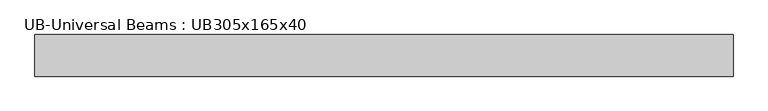
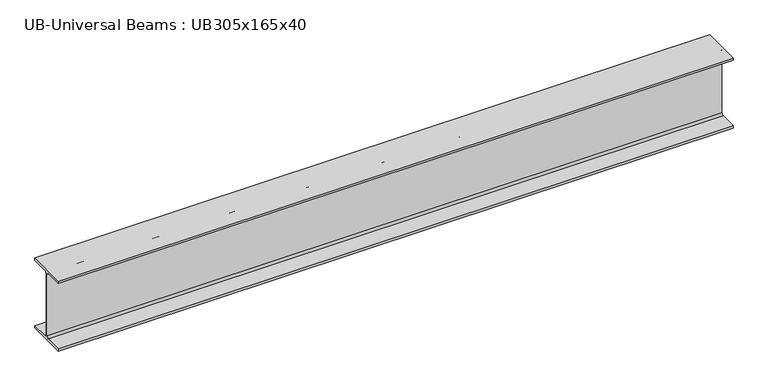
"""IFC4 building model written with IfcOpenShell, lengths in millimetres: beam geometry, UB-Universal Beams : UB305x165x40."""

from ifc_helpers import new_model, si_unit, point, frame, frame_2d, origin, place, context, project, spatial, polyline, circle_curve, trimmed, segment, composite_curve, outline, extrude, source, transform, mapped, element, save


def ub_universal_beams_ub305x165x40_b4961b4c(model_context):
    return source(origin(), model_context, "Body", "SweptSolid", [
        extrude(outline(composite_curve([segment(polyline([(82.5, -141.5), (82.5, -151.7), (-82.5, -151.7), (-82.5, -141.5), (-11.9, -141.5)]), True, "CONTINUOUS"), segment(trimmed(circle_curve(frame_2d((-11.9, -132.6)), 8.9), [point((-11.9, -141.5))], [point((-3.0, -132.6))], True, "CARTESIAN"), True, "CONTINUOUS"), segment(polyline([(-3.0, -132.6), (-3.0, 132.6)]), True, "CONTINUOUS"), segment(trimmed(circle_curve(frame_2d((-11.9, 132.6)), 8.9), [point((-3.0, 132.6))], [point((-11.9, 141.5))], True, "CARTESIAN"), True, "CONTINUOUS"), segment(polyline([(-11.9, 141.5), (-82.5, 141.5), (-82.5, 151.7), (82.5, 151.7), (82.5, 141.5), (11.9, 141.5)]), True, "CONTINUOUS"), segment(trimmed(circle_curve(frame_2d((11.9, 132.6)), 8.9), [point((11.9, 141.5))], [point((3.0, 132.6))], True, "CARTESIAN"), True, "CONTINUOUS"), segment(polyline([(3.0, 132.6), (3.0, -132.6)]), True, "CONTINUOUS"), segment(trimmed(circle_curve(frame_2d((11.9, -132.6)), 8.9), [point((3.0, -132.6))], [point((11.9, -141.5))], True, "CARTESIAN"), True, "CONTINUOUS"), segment(polyline([(11.9, -141.5), (82.5, -141.5)]), True, "CONTINUOUS")], self_intersect=False)), frame((-1439.45, 0.0, 0.0), z_axis=(1.0, 0.0, 0.0), x_axis=(0.0, 1.0, 0.0)), (0.0, 0.0, 1.0), 2765.0),
    ])


if __name__ == "__main__":
    model = new_model("IFC4")
    model_context = context("Model", 3, world=origin())
    ifc_project = project(units=[si_unit("LENGTHUNIT", "METRE", prefix="MILLI")], contexts=[model_context])
    site = spatial("IfcSite", under=ifc_project)
    building = spatial("IfcBuilding", under=site)
    placement = place(None, origin())
    ub_universal_beams_ub305x165x40_shape = ub_universal_beams_ub305x165x40_b4961b4c(model_context)
    element("IfcBeam", 1, ObjectType="UB-Universal Beams : UB305x165x40", at=placement, inside=building, context=model_context, shape_type="MappedRepresentation", body=[
        mapped(ub_universal_beams_ub305x165x40_shape, transform((0.0, 0.0, 0.0), x_axis=(1.0, 0.0, 0.0), y_axis=(0.0, 1.0, 0.0), z_axis=(0.0, 0.0, 1.0))),
    ])
    save(model, "model.ifc")

# Revit data of these elements
# Type "UB-Universal Beams : UB305x165x40"
#   Section Name Key = "UB305X165X40"
#   Width = 16.5 cm
#   Web Thickness = 0.6 cm
#   Web Fillet = 0.89 cm
#   Warping Constant = 164000.0 cm⁶
#   Torsional Moment of Inertia = 14.70 cm⁴
#   Section Area = 51.3 cm²
#   Plastic Modulus weak axis = 142.0 cm³
#   Plastic Modulus strong axis = 623.0 cm³
#   Nominal Weight = 40.2999 kgf/m
#   Moment of Inertia weak axis = 764.00 cm⁴
#   Moment of Inertia strong axis = 8503.00 cm⁴
#   Height = 30.34 cm
#   Flange Thickness = 1.02 cm
#   Elastic Modulus weak axis = 92.6 cm³
#   Elastic Modulus strong axis = 560.0 cm³
#   Centroid Vertical = 15.17 cm
#   Centroid Horizontal = 8.25 cm
#   Bolt Spacing = 9.0 cm
#   Length [instance default] = 1500 mm
#   Structural Material [instance default] = Metal - Steel 43-275
#   Type Comments = ""
#   Assembly Code = ""
# Element 1 (IfcBeam, "UB-Universal Beams : UB305x165x40")
#   Materials on its faces: "Metal - Steel 43-275"
# Materials
#   "Metal - Steel 43-275": class "Metal", colour RGB 247 247 247, transparency 0, Cost = 0
